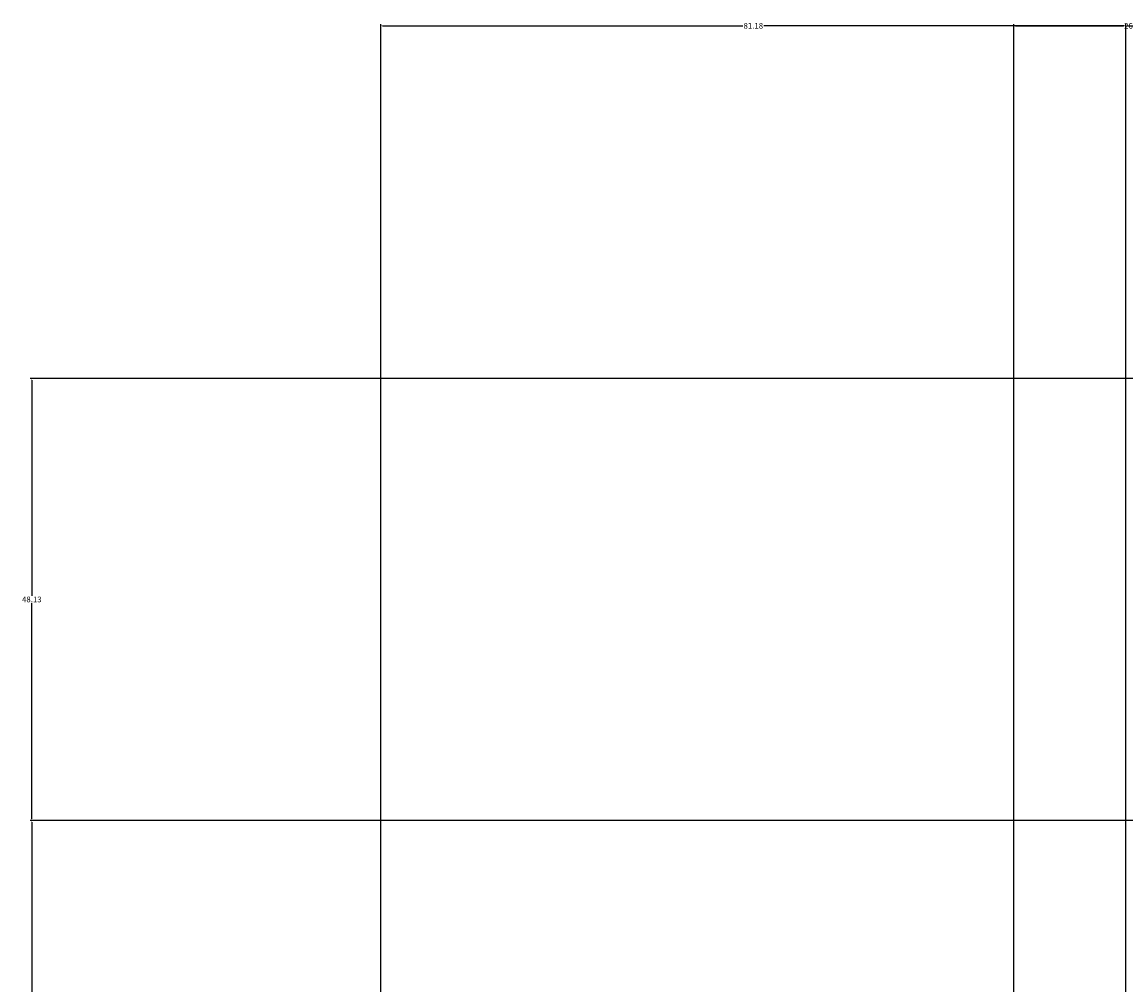
# Model space of a CAD drawing. Units: inches. Extents: x -13 to 809, y 112 to 656.
# Tile 28 of 55: x -13 to 107, y 551 to 656. Entities that reach past the tile are written whole.
import ezdxf

# ---------------------------------------------------------------- set-up
doc = ezdxf.new("R2010")
doc.units = ezdxf.units.IN
doc.header["$MEASUREMENT"] = 0
doc.layers.add('A-ANNO-DIMS', color=2, linetype='Continuous', lineweight=18)
doc.styles.get("Standard").update_dxf_attribs({"font": 'arial.ttf'})
doc.dimstyles.get("Standard").update_dxf_attribs({"dimtxt": 0.625, "dimasz": 0.18, "dimexe": 0.18, "dimexo": 0.0625, "dimgap": 0.09, "dimtad": 0, "dimtih": 1, "dimtoh": 1, "dimdec": 4, "dimzin": 0, "dimdsep": 46, "dimlunit": 4, "dimtxsty": 'Standard', "dimcen": 0.09, "dimadec": 0, "dimazin": 0, "dimtfac": 1, "dimtdec": 4, "dimtofl": 0, "dimtmove": 0, "dimatfit": 3, "dimfxl": 1, "dimtolj": 1, "dimtzin": 0, "dimarcsym": 0})

# ---------------------------------------------------------------- blocks, each defined once
blk = doc.blocks.new('*D22')
at = {"layer": 'A-ANNO-DIMS', "color": 0, "lineweight": -2, "transparency": 16777216}
for p, q in [((26.08, 210.58), (26.08, 655.96)), ((26.26, 655.78), (65.52, 655.78)), ((107.08, 655.78), (67.82, 655.78)), ((107.26, 510.58), (107.26, 655.96))]:
    blk.add_line(p, q, dxfattribs=at)
at = {"layer": 'A-ANNO-DIMS', "color": 0, "transparency": 16777216}
for points in [[(26.26, 655.81), (26.26, 655.75), (26.08, 655.78)], [(107.08, 655.81), (107.08, 655.75), (107.26, 655.78)]]:
    blk.add_solid(points, dxfattribs=at)
at = {"layer": 'Defpoints', "color": 0, "transparency": 16777216}
for p in [(107.26, 655.78), (107.26, 510.52), (26.08, 210.52)]:
    blk.add_point(p, dxfattribs=at)
at = {"layer": 'A-ANNO-DIMS', "color": 0, "transparency": 16777216, "insert": (66.67, 655.78), "char_height": 0.625, "attachment_point": 5}
blk.add_mtext('\\A1;81.18', dxfattribs=at)
blk = doc.blocks.new('*D23')
at = {"layer": 'A-ANNO-DIMS', "color": 0, "lineweight": -2, "transparency": 16777216}
for p, q in [((107.26, 510.58), (107.26, 655.96)), ((107.44, 655.78), (198.73, 655.78)), ((292.74, 655.78), (201.45, 655.78)), ((292.92, 569.3), (292.92, 655.96))]:
    blk.add_line(p, q, dxfattribs=at)
at = {"layer": 'A-ANNO-DIMS', "color": 0, "transparency": 16777216}
for points in [[(107.44, 655.81), (107.44, 655.75), (107.26, 655.78)], [(292.74, 655.81), (292.74, 655.75), (292.92, 655.78)]]:
    blk.add_solid(points, dxfattribs=at)
at = {"layer": 'Defpoints', "color": 0, "transparency": 16777216}
for p in [(292.92, 655.78), (292.92, 569.24), (107.26, 510.52)]:
    blk.add_point(p, dxfattribs=at)
at = {"layer": 'A-ANNO-DIMS', "color": 0, "transparency": 16777216, "insert": (200.09, 655.78), "char_height": 0.625, "attachment_point": 5}
blk.add_mtext('\\A1;185.66', dxfattribs=at)
blk = doc.blocks.new('*D36')
at = {"layer": 'A-ANNO-DIMS', "color": 0, "lineweight": -2, "transparency": 16777216}
for p, q in [((311.64, 569.24), (-12.1, 569.24)), ((-11.92, 569.06), (-11.92, 540.29)), ((-11.92, 510.7), (-11.92, 539.47)), ((107.2, 510.52), (-12.1, 510.52))]:
    blk.add_line(p, q, dxfattribs=at)
at = {"layer": 'A-ANNO-DIMS', "color": 0, "transparency": 16777216}
for points in [[(-11.95, 569.06), (-11.89, 569.06), (-11.92, 569.24)], [(-11.95, 510.7), (-11.89, 510.7), (-11.92, 510.52)]]:
    blk.add_solid(points, dxfattribs=at)
at = {"layer": 'Defpoints', "color": 0, "transparency": 16777216}
for p in [(-11.92, 569.24), (311.7, 569.24), (107.26, 510.52)]:
    blk.add_point(p, dxfattribs=at)
at = {"layer": 'A-ANNO-DIMS', "color": 0, "transparency": 16777216, "insert": (-11.92, 539.88), "char_height": 0.625, "attachment_point": 5}
blk.add_mtext('\\A1;58.72', dxfattribs=at)
blk = doc.blocks.new('*D37')
at = {"layer": 'A-ANNO-DIMS', "color": 0, "lineweight": -2, "transparency": 16777216}
for p, q in [((311.64, 617.37), (-12.1, 617.37)), ((-11.92, 617.19), (-11.92, 593.72)), ((-11.92, 569.42), (-11.92, 592.9)), ((311.64, 569.24), (-12.1, 569.24))]:
    blk.add_line(p, q, dxfattribs=at)
at = {"layer": 'A-ANNO-DIMS', "color": 0, "transparency": 16777216}
for points in [[(-11.95, 617.19), (-11.89, 617.19), (-11.92, 617.37)], [(-11.95, 569.42), (-11.89, 569.42), (-11.92, 569.24)]]:
    blk.add_solid(points, dxfattribs=at)
at = {"layer": 'Defpoints', "color": 0, "transparency": 16777216}
for p in [(-11.92, 617.37), (311.7, 617.37), (311.7, 569.24)]:
    blk.add_point(p, dxfattribs=at)
at = {"layer": 'A-ANNO-DIMS', "color": 0, "transparency": 16777216, "insert": (-11.92, 593.31), "char_height": 0.625, "attachment_point": 5}
blk.add_mtext('\\A1;48.13', dxfattribs=at)
blk = doc.blocks.new('*D95')
at = {"layer": 'A-ANNO-DIMS', "color": 0, "lineweight": -2, "transparency": 16777216}
for p, q in [((95.05, 462.58), (95.05, 655.96)), ((95.23, 655.78), (106.98, 655.78)), ((121.02, 655.78), (109.28, 655.78)), ((121.2, 452.63), (121.2, 655.96))]:
    blk.add_line(p, q, dxfattribs=at)
at = {"layer": 'A-ANNO-DIMS', "color": 0, "transparency": 16777216}
for points in [[(95.23, 655.81), (95.23, 655.75), (95.05, 655.78)], [(121.02, 655.81), (121.02, 655.75), (121.2, 655.78)]]:
    blk.add_solid(points, dxfattribs=at)
at = {"layer": 'Defpoints', "color": 0, "transparency": 16777216}
for p in [(121.2, 655.78), (95.05, 462.52), (121.2, 452.56)]:
    blk.add_point(p, dxfattribs=at)
at = {"layer": 'A-ANNO-DIMS', "color": 0, "transparency": 16777216, "insert": (108.13, 655.78), "char_height": 0.625, "attachment_point": 5}
blk.add_mtext('\\A1;26.16', dxfattribs=at)

msp = doc.modelspace()

# ---------------------------------------------------------------- dimensions: what is measured, and where the dimension line sits
at = {"layer": 'A-ANNO-DIMS'}
for base, p1, p2, picture, middle in [((107.2588, 655.7828), (26.0809, 210.5199), (107.2588, 510.5199), '*D22', (66.6698, 655.7828)), ((121.2048, 655.7828), (95.0469, 462.5199), (121.2048, 452.5629), '*D95', (108.1258, 655.7828)), ((292.923, 655.7828), (107.2588, 510.5199), (292.923, 569.2414), '*D23', (200.0909, 655.7828))]:
    dim = msp.add_linear_dim(base=base, p1=p1, p2=p2, dimstyle='Standard', override={"dimdec": 2, "dimlfac": 1, "dimrnd": 0, "dimzin": 0, "dimdsep": 46, "dimlunit": 2}, dxfattribs=at)
    dim.commit()
    dim.dimension.update_dxf_attribs({"geometry": picture, "text_midpoint": middle})
for base, p1, p2, picture, middle in [((-11.9191, 617.3708), (311.6991, 569.2414), (311.6991, 617.3708), '*D37', (-11.9191, 593.3061)), ((-11.9191, 569.2414), (107.2588, 510.5199), (311.6991, 569.2414), '*D36', (-11.9191, 539.8806))]:
    dim = msp.add_linear_dim(base=base, p1=p1, p2=p2, angle=90, dimstyle='Standard', override={"dimdec": 2, "dimlfac": 1, "dimrnd": 0, "dimzin": 0, "dimdsep": 46, "dimlunit": 2}, dxfattribs=at)
    dim.commit()
    dim.dimension.update_dxf_attribs({"geometry": picture, "text_midpoint": middle})

doc.saveas('drawing.dxf')
